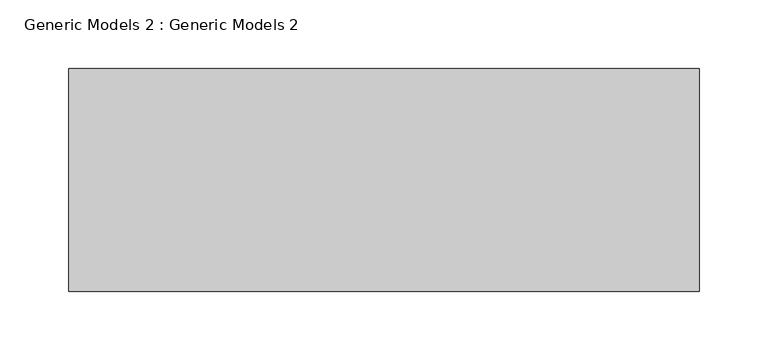
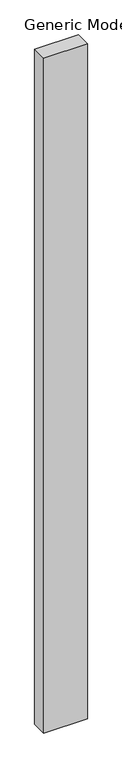
"""IFC4 building model written with IfcOpenShell, lengths in millimetres: proxy geometry, Generic Models 2 : Generic Models 2."""

from ifc_helpers import new_model, si_unit, frame, origin, place, context, project, spatial, polyline, outline, extrude, source, transform, mapped, element, save


def generic_models_2_generic_models_2_c6cf683d(model_context):
    return source(origin(), model_context, "Body", "SweptSolid", [
        extrude(outline(polyline([(-13097.1551496, -2047.6916291), (-13554.3551496, -2047.6916291), (-13554.3551496, -1885.997359), (-13097.1551496, -1885.997359), (-13097.1551496, -2047.6916291)])), frame((0.0, 0.0, -152.4), z_axis=(0.0, 0.0, 1.0), x_axis=(1.0, 0.0, 0.0)), (0.0, 0.0, 1.0), 7467.6),
    ])


if __name__ == "__main__":
    model = new_model("IFC4")
    model_context = context("Model", 3, world=origin())
    ifc_project = project(units=[si_unit("LENGTHUNIT", "METRE", prefix="MILLI")], contexts=[model_context])
    site = spatial("IfcSite", under=ifc_project)
    building = spatial("IfcBuilding", under=site)
    placement = place(None, origin())
    generic_models_2_generic_models_2_shape = generic_models_2_generic_models_2_c6cf683d(model_context)
    element("IfcBuildingElementProxy", 1, Name="Generic Models 2 : Generic Models 2", ObjectType="Generic Models 2 : Generic Models 2", at=placement, inside=building, context=model_context, shape_type="MappedRepresentation", body=[
        mapped(generic_models_2_generic_models_2_shape, transform((0.0, 0.0, 0.0), x_axis=(1.0, 0.0, 0.0), y_axis=(0.0, 1.0, 0.0), z_axis=(0.0, 0.0, 1.0))),
    ])
    save(model, "model.ifc")
